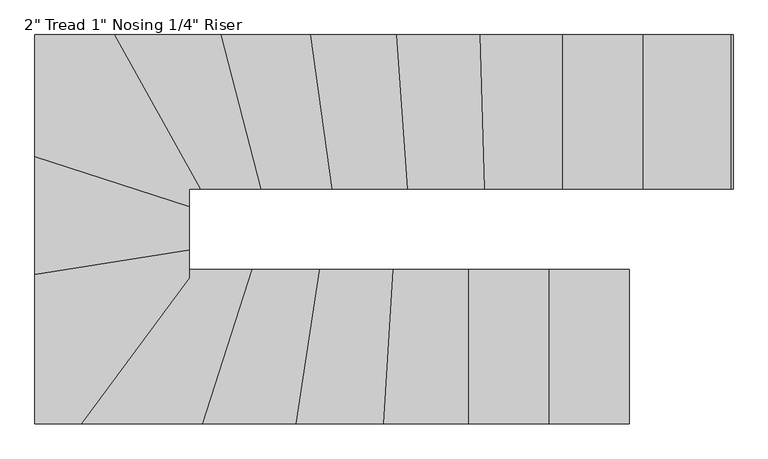
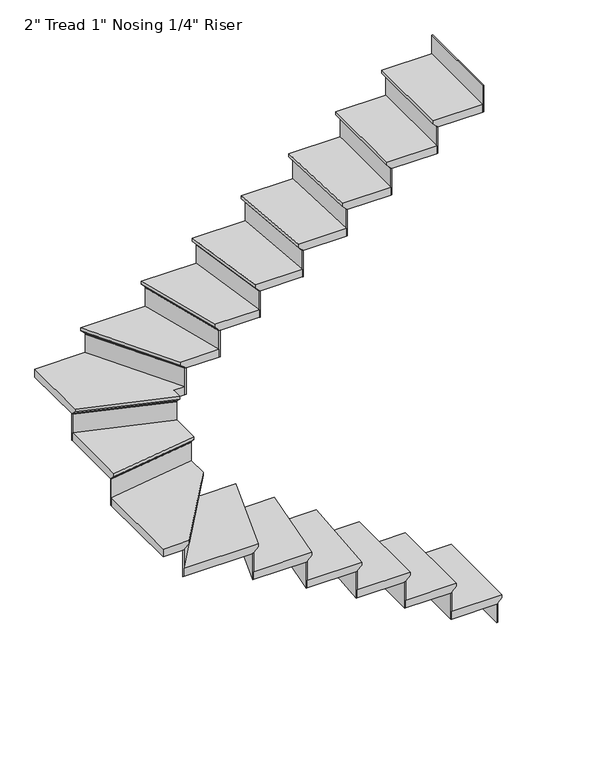
"""IFC4 building model written with IfcOpenShell, lengths in millimetres: stair flight geometry."""

from ifc_helpers import new_model, si_unit, origin, place, context, project, spatial, faceted_brep, source, transform, mapped, element, save


def stair_flight_0735e5f0(model_context):
    return source(origin(), model_context, "Body", "Brep", [
        faceted_brep([(-264.8831579, 264.4433073, 150.2833333), (-264.8831579, 264.4433073, 169.3333333), (-264.8831579, -271.8029286, 169.3333333), (-264.8831579, -271.8029286, 150.2833333), (-290.2831579, 264.4433073, 124.8833333), (-290.2831579, -271.8029286, 124.8833333), (-569.6831579, 264.4433073, 169.3333333), (-569.6831579, -271.8029286, 169.3333333), (-290.2831579, -271.8029286, 118.5333333), (-569.6831579, -271.8029286, 118.5333333), (-569.6831579, 264.4433073, 118.5333333), (-290.2831579, 264.4433073, 118.5333333)], [[[0, 1, 2, 3]], [[4, 0, 3, 5]], [[2, 1, 6, 7]], [[8, 9, 10, 11]], [[2, 7, 9, 8, 5, 3]], [[8, 11, 4, 5]], [[6, 1, 0, 4, 11, 10]], [[7, 6, 10, 9]]]),
        faceted_brep([(-290.2831579, 264.4433073, 118.5333333), (-290.2831579, 264.4433073, 0.0), (-296.6331579, 264.4433073, 0.0), (-296.6331579, 264.4433073, 118.5333333), (-290.2831579, -271.8029286, 118.5333333), (-296.6331579, -271.8029286, 118.5333333), (-296.6331579, -271.8029286, 0.0), (-290.2831579, -271.8029286, 0.0)], [[[0, 1, 2, 3]], [[4, 5, 6, 7]], [[1, 0, 4, 7]], [[2, 1, 7, 6]], [[3, 2, 6, 5]], [[0, 3, 5, 4]]]),
        faceted_brep([(-569.6831579, 264.4433073, 287.8666667), (-569.6831579, 264.4433073, 118.5333333), (-576.0331579, 264.4433073, 118.5333333), (-576.0331579, 264.4433073, 287.8666667), (-569.6831579, -271.8029286, 287.8666667), (-576.0331579, -271.8029286, 287.8666667), (-576.0331579, -271.8029286, 118.5333333), (-569.6831579, -271.8029286, 118.5333333)], [[[0, 1, 2, 3]], [[4, 5, 6, 7]], [[1, 0, 4, 7]], [[2, 1, 7, 6]], [[3, 2, 6, 5]], [[0, 3, 5, 4]]]),
        faceted_brep([(-544.2831579, -271.8029286, 338.6666667), (-544.2831579, 264.4433073, 338.6666667), (-849.0831579, 264.4433073, 338.6666667), (-849.0831579, -271.8029286, 338.6666667), (-569.6831579, -271.8029286, 287.8666667), (-849.0831579, -271.8029286, 287.8666667), (-849.0831579, 264.4433073, 287.8666667), (-569.6831579, 264.4433073, 287.8666667), (-569.6831579, -271.8029286, 294.2166667), (-544.2831579, -271.8029286, 319.6166667), (-569.6831579, 264.4433073, 294.2166667), (-544.2831579, 264.4433073, 319.6166667)], [[[0, 1, 2, 3]], [[4, 5, 6, 7]], [[0, 3, 5, 4, 8, 9]], [[4, 7, 10, 8]], [[2, 1, 11, 10, 7, 6]], [[3, 2, 6, 5]], [[11, 1, 0, 9]], [[10, 11, 9, 8]]]),
        faceted_brep([(-849.0831579, 264.4433073, 457.2), (-849.0831579, 264.4433073, 287.8666667), (-855.4331579, 264.4433073, 287.8666667), (-855.4331579, 264.4433073, 457.2), (-849.0831579, -271.8029286, 457.2), (-855.4331579, -271.8029286, 457.2), (-855.4331579, -271.8029286, 287.8666667), (-849.0831579, -271.8029286, 287.8666667)], [[[0, 1, 2, 3]], [[4, 5, 6, 7]], [[1, 0, 4, 7]], [[2, 1, 7, 6]], [[3, 2, 6, 5]], [[0, 3, 5, 4]]]),
        faceted_brep([(-823.6831579, -271.8029286, 508.0), (-823.6831579, 264.4433073, 508.0), (-1112.6009003, 264.4433073, 508.0), (-1144.4549627, -271.8029286, 508.0), (-849.0831579, -271.8029286, 457.2), (-1144.4549627, -271.8029286, 457.2), (-1112.6009003, 264.4433073, 457.2), (-849.0831579, 264.4433073, 457.2), (-849.0831579, -271.8029286, 463.55), (-823.6831579, -271.8029286, 488.95), (-849.0831579, 264.4433073, 463.55), (-823.6831579, 264.4433073, 488.95)], [[[0, 1, 2, 3]], [[4, 5, 6, 7]], [[0, 3, 5, 4, 8, 9]], [[4, 7, 10, 8]], [[2, 1, 11, 10, 7, 6]], [[3, 2, 6, 5]], [[11, 1, 0, 9]], [[10, 11, 9, 8]]]),
        faceted_brep([(-1112.6009003, 264.4433073, 626.5333333), (-1112.6009003, 264.4433073, 457.2), (-1118.9620938, 264.4433073, 457.2), (-1118.9620938, 264.4433073, 626.5333333), (-1144.4549627, -271.8029286, 626.5333333), (-1150.8161561, -271.8029286, 626.5333333), (-1150.8161561, -271.8029286, 457.2), (-1144.4549627, -271.8029286, 457.2)], [[[0, 1, 2, 3]], [[4, 5, 6, 7]], [[1, 0, 4, 7]], [[2, 1, 7, 6]], [[3, 2, 6, 5]], [[0, 3, 5, 4]]]),
        faceted_brep([(-1119.0101891, -271.8029286, 677.3333333), (-1087.1561267, 264.4433073, 677.3333333), (-1367.1376579, 264.4433073, 677.3333333), (-1449.2203373, -271.8029286, 677.3333333), (-1144.4549627, -271.8029286, 626.5333333), (-1449.2203373, -271.8029286, 626.5333333), (-1367.1376579, 264.4433073, 626.5333333), (-1112.6009003, 264.4433073, 626.5333333), (-1144.4549627, -271.8029286, 632.8833333), (-1119.0101891, -271.8029286, 658.2833333), (-1112.6009003, 264.4433073, 632.8833333), (-1087.1561267, 264.4433073, 658.2833333)], [[[0, 1, 2, 3]], [[4, 5, 6, 7]], [[0, 3, 5, 4, 8, 9]], [[4, 7, 10, 8]], [[2, 1, 11, 10, 7, 6]], [[3, 2, 6, 5]], [[11, 1, 0, 9]], [[10, 11, 9, 8]]]),
        faceted_brep([(-1367.1376579, 264.4433073, 795.8666667), (-1367.1376579, 264.4433073, 626.5333333), (-1373.5616178, 264.4433073, 626.5333333), (-1373.5616178, 264.4433073, 795.8666667), (-1449.2203373, -271.8029286, 795.8666667), (-1455.6442972, -271.8029286, 795.8666667), (-1455.6442972, -271.8029286, 626.5333333), (-1449.2203373, -271.8029286, 626.5333333)], [[[0, 1, 2, 3]], [[4, 5, 6, 7]], [[1, 0, 4, 7]], [[2, 1, 7, 6]], [[3, 2, 6, 5]], [[0, 3, 5, 4]]]),
        faceted_brep([(-1423.5244976, -271.8029286, 846.6666667), (-1341.4418182, 264.4433073, 846.6666667), (-1602.0584075, 264.4433073, 846.6666667), (-1775.0869242, -271.8029286, 846.6666667), (-1449.2203373, -271.8029286, 795.8666667), (-1775.0869242, -271.8029286, 795.8666667), (-1602.0584075, 264.4433073, 795.8666667), (-1367.1376579, 264.4433073, 795.8666667), (-1449.2203373, -271.8029286, 802.2166667), (-1423.5244976, -271.8029286, 827.6166667), (-1367.1376579, 264.4433073, 802.2166667), (-1341.4418182, 264.4433073, 827.6166667)], [[[0, 1, 2, 3]], [[4, 5, 6, 7]], [[0, 3, 5, 4, 8, 9]], [[4, 7, 10, 8]], [[2, 1, 11, 10, 7, 6]], [[3, 2, 6, 5]], [[11, 1, 0, 9]], [[10, 11, 9, 8]]]),
        faceted_brep([(-1602.0584075, 264.4433073, 965.2), (-1602.0584075, 264.4433073, 795.8666667), (-1608.7307845, 264.4433073, 795.8666667), (-1608.7307845, 264.4433073, 965.2), (-1775.0869242, -271.8029286, 965.2), (-1781.7593012, -271.8029286, 965.2), (-1781.7593012, -271.8029286, 795.8666667), (-1775.0869242, -271.8029286, 795.8666667)], [[[0, 1, 2, 3]], [[4, 5, 6, 7]], [[1, 0, 4, 7]], [[2, 1, 7, 6]], [[3, 2, 6, 5]], [[0, 3, 5, 4]]]),
        faceted_brep([(-1748.3974163, -271.8029286, 1016.0), (-1575.3688995, 264.4433073, 1016.0), (-1792.6148498, 264.4433073, 1016.0), (-1792.6148498, 277.721026, 1016.0), (-2200.2950016, -271.8029286, 1016.0), (-1775.0869242, -271.8029286, 965.2), (-2200.2950016, -271.8029286, 965.2), (-1792.6148498, 277.721026, 965.2), (-1792.6148498, 264.4433073, 965.2), (-1602.0584075, 264.4433073, 965.2), (-1775.0869242, -271.8029286, 971.55), (-1748.3974163, -271.8029286, 996.95), (-1602.0584075, 264.4433073, 971.55), (-1575.3688995, 264.4433073, 996.95)], [[[0, 1, 2, 3, 4]], [[5, 6, 7, 8, 9]], [[0, 4, 6, 5, 10, 11]], [[5, 9, 12, 10]], [[2, 1, 13, 12, 9, 8]], [[4, 3, 7, 6]], [[13, 1, 0, 11]], [[12, 13, 11, 10]], [[3, 2, 8, 7]]]),
        faceted_brep([(-1792.6148498, 277.721026, 1134.5333333), (-1792.6148498, 277.721026, 965.2), (-1792.6148498, 288.3786511, 965.2), (-1792.6148498, 288.3786511, 1134.5333333), (-2200.2950016, -271.8029286, 1134.5333333), (-2208.2016673, -271.8029286, 1134.5333333), (-2208.2016673, -271.8029286, 965.2), (-2200.2950016, -271.8029286, 965.2)], [[[0, 1, 2, 3]], [[4, 5, 6, 7]], [[1, 0, 4, 7]], [[2, 1, 7, 6]], [[3, 2, 6, 5]], [[0, 3, 5, 4]]]),
        faceted_brep([(-2328.8610857, 272.9225747, 1185.3333333), (-2328.8610857, -271.8029286, 1185.3333333), (-2168.6683387, -271.8029286, 1185.3333333), (-1792.6148498, 235.0905257, 1185.3333333), (-1792.6148498, 358.7948785, 1185.3333333), (-2328.8610857, -271.8029286, 1134.5333333), (-2328.8610857, 272.9225747, 1134.5333333), (-1792.6148498, 358.7948785, 1134.5333333), (-1792.6148498, 277.721026, 1134.5333333), (-2200.2950016, -271.8029286, 1134.5333333), (-2200.2950016, -271.8029286, 1140.8833333), (-2168.6683387, -271.8029286, 1166.2833333), (-1792.6148498, 277.721026, 1140.8833333), (-1792.6148498, 235.0905257, 1166.2833333)], [[[0, 1, 2, 3, 4]], [[5, 6, 7, 8, 9]], [[1, 0, 6, 5]], [[2, 1, 5, 9, 10, 11]], [[9, 8, 12, 10]], [[4, 3, 13, 12, 8, 7]], [[0, 4, 7, 6]], [[13, 3, 2, 11]], [[12, 13, 11, 10]]]),
        faceted_brep([(-1792.6148498, 358.7948785, 1303.8666667), (-1792.6148498, 358.7948785, 1134.5333333), (-1792.6148498, 365.2257813, 1134.5333333), (-1792.6148498, 365.2257813, 1303.8666667), (-2328.8610857, 272.9225747, 1303.8666667), (-2328.8610857, 279.3534775, 1303.8666667), (-2328.8610857, 279.3534775, 1134.5333333), (-2328.8610857, 272.9225747, 1134.5333333)], [[[0, 1, 2, 3]], [[4, 5, 6, 7]], [[1, 0, 4, 7]], [[2, 1, 7, 6]], [[3, 2, 6, 5]], [[0, 3, 5, 4]]]),
        faceted_brep([(-2328.8610857, 247.1989634, 1354.6666667), (-1792.6148498, 333.0712672, 1354.6666667), (-1792.6148498, 510.0383883, 1354.6666667), (-2328.8610857, 683.2061106, 1354.6666667), (-2328.8610857, 272.9225747, 1303.8666667), (-2328.8610857, 683.2061106, 1303.8666667), (-1792.6148498, 510.0383883, 1303.8666667), (-1792.6148498, 358.7948785, 1303.8666667), (-2328.8610857, 272.9225747, 1310.2166667), (-2328.8610857, 247.1989634, 1335.6166667), (-1792.6148498, 358.7948785, 1310.2166667), (-1792.6148498, 333.0712672, 1335.6166667)], [[[0, 1, 2, 3]], [[4, 5, 6, 7]], [[0, 3, 5, 4, 8, 9]], [[4, 7, 10, 8]], [[3, 2, 6, 5]], [[11, 1, 0, 9]], [[10, 11, 9, 8]], [[2, 1, 11, 10, 7, 6]]]),
        faceted_brep([(-1792.6148498, 510.0383883, 1473.2), (-1792.6148498, 510.0383883, 1303.8666667), (-1792.6148498, 516.7112716, 1303.8666667), (-1792.6148498, 516.7112716, 1473.2), (-2328.8610857, 683.2061106, 1473.2), (-2328.8610857, 689.878994, 1473.2), (-2328.8610857, 689.878994, 1303.8666667), (-2328.8610857, 683.2061106, 1303.8666667)], [[[0, 1, 2, 3]], [[4, 5, 6, 7]], [[1, 0, 4, 7]], [[2, 1, 7, 6]], [[3, 2, 6, 5]], [[0, 3, 5, 4]]]),
        faceted_brep([(-2021.9568272, 1080.0895433, 1524.0), (-2328.8610857, 1080.0895433, 1524.0), (-2328.8610857, 656.5145772, 1524.0), (-1792.6148498, 483.3468548, 1524.0), (-1792.6148498, 543.8433073, 1524.0), (-1724.5287393, 543.8433073, 1524.0), (-2328.8610857, 1080.0895433, 1473.2), (-2021.9568272, 1080.0895433, 1473.2), (-1724.5287393, 543.8433073, 1473.2), (-1792.6148498, 543.8433073, 1473.2), (-1792.6148498, 510.0383883, 1473.2), (-2328.8610857, 683.2061106, 1473.2), (-1792.6148498, 510.0383883, 1479.55), (-2328.8610857, 683.2061106, 1479.55), (-1792.6148498, 483.3468548, 1504.95), (-2328.8610857, 656.5145772, 1504.95)], [[[0, 1, 2, 3, 4, 5]], [[6, 7, 8, 9, 10, 11]], [[1, 0, 7, 6]], [[11, 10, 12, 13]], [[4, 3, 14, 12, 10, 9]], [[0, 5, 8, 7]], [[14, 3, 2, 15]], [[12, 14, 15, 13]], [[2, 1, 6, 11, 13, 15]], [[5, 4, 9, 8]]]),
        faceted_brep([(-1724.5287393, 543.8433073, 1642.5333333), (-1724.5287393, 543.8433073, 1473.2), (-1717.2673962, 543.8433073, 1473.2), (-1717.2673962, 543.8433073, 1642.5333333), (-2021.9568272, 1080.0895433, 1642.5333333), (-2014.6954841, 1080.0895433, 1642.5333333), (-2014.6954841, 1080.0895433, 1473.2), (-2021.9568272, 1080.0895433, 1473.2)], [[[0, 1, 2, 3]], [[4, 5, 6, 7]], [[1, 0, 4, 7]], [[2, 1, 7, 6]], [[3, 2, 6, 5]], [[0, 3, 5, 4]]]),
        faceted_brep([(-2051.0021996, 1080.0895433, 1693.3333333), (-1753.5741117, 543.8433073, 1693.3333333), (-1517.487325, 543.8433073, 1693.3333333), (-1656.0375972, 1080.0895433, 1693.3333333), (-2021.9568272, 1080.0895433, 1642.5333333), (-1656.0375972, 1080.0895433, 1642.5333333), (-1517.487325, 543.8433073, 1642.5333333), (-1724.5287393, 543.8433073, 1642.5333333), (-2021.9568272, 1080.0895433, 1648.8833333), (-2051.0021996, 1080.0895433, 1674.2833333), (-1724.5287393, 543.8433073, 1648.8833333), (-1753.5741117, 543.8433073, 1674.2833333)], [[[0, 1, 2, 3]], [[4, 5, 6, 7]], [[0, 3, 5, 4, 8, 9]], [[4, 7, 10, 8]], [[2, 1, 11, 10, 7, 6]], [[3, 2, 6, 5]], [[11, 1, 0, 9]], [[10, 11, 9, 8]]]),
        faceted_brep([(-1517.487325, 543.8433073, 1811.8666667), (-1517.487325, 543.8433073, 1642.5333333), (-1510.9288005, 543.8433073, 1642.5333333), (-1510.9288005, 543.8433073, 1811.8666667), (-1656.0375972, 1080.0895433, 1811.8666667), (-1649.4790727, 1080.0895433, 1811.8666667), (-1649.4790727, 1080.0895433, 1642.5333333), (-1656.0375972, 1080.0895433, 1642.5333333)], [[[0, 1, 2, 3]], [[4, 5, 6, 7]], [[1, 0, 4, 7]], [[2, 1, 7, 6]], [[3, 2, 6, 5]], [[0, 3, 5, 4]]]),
        faceted_brep([(-1682.2716952, 1080.0895433, 1862.6666667), (-1543.721423, 543.8433073, 1862.6666667), (-1271.2041837, 543.8433073, 1862.6666667), (-1344.713853, 1080.0895433, 1862.6666667), (-1656.0375972, 1080.0895433, 1811.8666667), (-1344.713853, 1080.0895433, 1811.8666667), (-1271.2041837, 543.8433073, 1811.8666667), (-1517.487325, 543.8433073, 1811.8666667), (-1656.0375972, 1080.0895433, 1818.2166667), (-1682.2716952, 1080.0895433, 1843.6166667), (-1517.487325, 543.8433073, 1818.2166667), (-1543.721423, 543.8433073, 1843.6166667)], [[[0, 1, 2, 3]], [[4, 5, 6, 7]], [[0, 3, 5, 4, 8, 9]], [[4, 7, 10, 8]], [[2, 1, 11, 10, 7, 6]], [[3, 2, 6, 5]], [[11, 1, 0, 9]], [[10, 11, 9, 8]]]),
        faceted_brep([(-1271.2041837, 543.8433073, 1981.2), (-1271.2041837, 543.8433073, 1811.8666667), (-1264.7947985, 543.8433073, 1811.8666667), (-1264.7947985, 543.8433073, 1981.2), (-1344.713853, 1080.0895433, 1981.2), (-1338.3044678, 1080.0895433, 1981.2), (-1338.3044678, 1080.0895433, 1811.8666667), (-1344.713853, 1080.0895433, 1811.8666667)], [[[0, 1, 2, 3]], [[4, 5, 6, 7]], [[1, 0, 4, 7]], [[2, 1, 7, 6]], [[3, 2, 6, 5]], [[0, 3, 5, 4]]]),
        faceted_brep([(-1370.3513937, 1080.0895433, 2032.0), (-1296.8417245, 543.8433073, 2032.0), (-1009.7763573, 543.8433073, 2032.0), (-1047.6899509, 1080.0895433, 2032.0), (-1344.713853, 1080.0895433, 1981.2), (-1047.6899509, 1080.0895433, 1981.2), (-1009.7763573, 543.8433073, 1981.2), (-1271.2041837, 543.8433073, 1981.2), (-1344.713853, 1080.0895433, 1987.55), (-1370.3513937, 1080.0895433, 2012.95), (-1271.2041837, 543.8433073, 1987.55), (-1296.8417245, 543.8433073, 2012.95)], [[[0, 1, 2, 3]], [[4, 5, 6, 7]], [[0, 3, 5, 4, 8, 9]], [[4, 7, 10, 8]], [[2, 1, 11, 10, 7, 6]], [[3, 2, 6, 5]], [[11, 1, 0, 9]], [[10, 11, 9, 8]]]),
        faceted_brep([(-1009.7763573, 543.8433073, 2150.5333333), (-1009.7763573, 543.8433073, 1981.2), (-1003.4105061, 543.8433073, 1981.2), (-1003.4105061, 543.8433073, 2150.5333333), (-1047.6899509, 1080.0895433, 2150.5333333), (-1041.3240997, 1080.0895433, 2150.5333333), (-1041.3240997, 1080.0895433, 1981.2), (-1047.6899509, 1080.0895433, 1981.2)], [[[0, 1, 2, 3]], [[4, 5, 6, 7]], [[1, 0, 4, 7]], [[2, 1, 7, 6]], [[3, 2, 6, 5]], [[0, 3, 5, 4]]]),
        faceted_brep([(-1073.1533559, 1080.0895433, 2201.3333333), (-1035.2397623, 543.8433073, 2201.3333333), (-741.6570892, 543.8433073, 2201.3333333), (-757.1149275, 1080.0895433, 2201.3333333), (-1047.6899509, 1080.0895433, 2150.5333333), (-757.1149275, 1080.0895433, 2150.5333333), (-741.6570892, 543.8433073, 2150.5333333), (-1009.7763573, 543.8433073, 2150.5333333), (-1047.6899509, 1080.0895433, 2156.8833333), (-1073.1533559, 1080.0895433, 2182.2833333), (-1009.7763573, 543.8433073, 2156.8833333), (-1035.2397623, 543.8433073, 2182.2833333)], [[[0, 1, 2, 3]], [[4, 5, 6, 7]], [[0, 3, 5, 4, 8, 9]], [[4, 7, 10, 8]], [[2, 1, 11, 10, 7, 6]], [[3, 2, 6, 5]], [[11, 1, 0, 9]], [[10, 11, 9, 8]]]),
        faceted_brep([(-741.6570892, 543.8433073, 2319.8666667), (-741.6570892, 543.8433073, 2150.5333333), (-735.3044516, 543.8433073, 2150.5333333), (-735.3044516, 543.8433073, 2319.8666667), (-757.1149275, 1080.0895433, 2319.8666667), (-750.7622898, 1080.0895433, 2319.8666667), (-750.7622898, 1080.0895433, 2150.5333333), (-757.1149275, 1080.0895433, 2150.5333333)], [[[0, 1, 2, 3]], [[4, 5, 6, 7]], [[1, 0, 4, 7]], [[2, 1, 7, 6]], [[3, 2, 6, 5]], [[0, 3, 5, 4]]]),
        faceted_brep([(-782.5254783, 1080.0895433, 2370.6666667), (-767.06764, 543.8433073, 2370.6666667), (-469.9965591, 543.8433073, 2370.6666667), (-469.9965591, 1080.0895433, 2370.6666667), (-757.1149275, 1080.0895433, 2319.8666667), (-469.9965591, 1080.0895433, 2319.8666667), (-469.9965591, 543.8433073, 2319.8666667), (-741.6570892, 543.8433073, 2319.8666667), (-757.1149275, 1080.0895433, 2326.2166667), (-782.5254783, 1080.0895433, 2351.6166667), (-741.6570892, 543.8433073, 2326.2166667), (-767.06764, 543.8433073, 2351.6166667)], [[[0, 1, 2, 3]], [[4, 5, 6, 7]], [[0, 3, 5, 4, 8, 9]], [[4, 7, 10, 8]], [[2, 1, 11, 10, 7, 6]], [[3, 2, 6, 5]], [[11, 1, 0, 9]], [[10, 11, 9, 8]]]),
        faceted_brep([(-469.9965591, 543.8433073, 2489.2), (-469.9965591, 543.8433073, 2319.8666667), (-463.6465591, 543.8433073, 2319.8666667), (-463.6465591, 543.8433073, 2489.2), (-469.9965591, 1080.0895433, 2489.2), (-463.6465591, 1080.0895433, 2489.2), (-463.6465591, 1080.0895433, 2319.8666667), (-469.9965591, 1080.0895433, 2319.8666667)], [[[0, 1, 2, 3]], [[4, 5, 6, 7]], [[1, 0, 4, 7]], [[2, 1, 7, 6]], [[3, 2, 6, 5]], [[0, 3, 5, 4]]]),
        faceted_brep([(-495.3965591, 1080.0895433, 2540.0), (-495.3965591, 543.8433073, 2540.0), (-190.5965591, 543.8433073, 2540.0), (-190.5965591, 1080.0895433, 2540.0), (-469.9965591, 1080.0895433, 2489.2), (-190.5965591, 1080.0895433, 2489.2), (-190.5965591, 543.8433073, 2489.2), (-469.9965591, 543.8433073, 2489.2), (-469.9965591, 1080.0895433, 2495.55), (-495.3965591, 1080.0895433, 2520.95), (-469.9965591, 543.8433073, 2495.55), (-495.3965591, 543.8433073, 2520.95)], [[[0, 1, 2, 3]], [[4, 5, 6, 7]], [[0, 3, 5, 4, 8, 9]], [[4, 7, 10, 8]], [[2, 1, 11, 10, 7, 6]], [[3, 2, 6, 5]], [[11, 1, 0, 9]], [[10, 11, 9, 8]]]),
        faceted_brep([(-190.5965591, 543.8433073, 2658.5333333), (-190.5965591, 543.8433073, 2489.2), (-184.2465591, 543.8433073, 2489.2), (-184.2465591, 543.8433073, 2658.5333333), (-190.5965591, 1080.0895433, 2658.5333333), (-184.2465591, 1080.0895433, 2658.5333333), (-184.2465591, 1080.0895433, 2489.2), (-190.5965591, 1080.0895433, 2489.2)], [[[0, 1, 2, 3]], [[4, 5, 6, 7]], [[1, 0, 4, 7]], [[2, 1, 7, 6]], [[3, 2, 6, 5]], [[0, 3, 5, 4]]]),
        faceted_brep([(88.8034409, 543.8433073, 2827.8666667), (88.8034409, 543.8433073, 2658.5333333), (95.1534409, 543.8433073, 2658.5333333), (95.1534409, 543.8433073, 2827.8666667), (88.8034409, 1080.0895433, 2827.8666667), (95.1534409, 1080.0895433, 2827.8666667), (95.1534409, 1080.0895433, 2658.5333333), (88.8034409, 1080.0895433, 2658.5333333)], [[[0, 1, 2, 3]], [[4, 5, 6, 7]], [[1, 0, 4, 7]], [[2, 1, 7, 6]], [[3, 2, 6, 5]], [[0, 3, 5, 4]]]),
        faceted_brep([(-215.9965591, 1080.0895433, 2709.3333333), (-215.9965591, 543.8433073, 2709.3333333), (88.8034409, 543.8433073, 2709.3333333), (88.8034409, 1080.0895433, 2709.3333333), (-190.5965591, 1080.0895433, 2658.5333333), (88.8034409, 1080.0895433, 2658.5333333), (88.8034409, 543.8433073, 2658.5333333), (-190.5965591, 543.8433073, 2658.5333333), (-190.5965591, 1080.0895433, 2664.8833333), (-215.9965591, 1080.0895433, 2690.2833333), (-190.5965591, 543.8433073, 2664.8833333), (-215.9965591, 543.8433073, 2690.2833333)], [[[0, 1, 2, 3]], [[4, 5, 6, 7]], [[0, 3, 5, 4, 8, 9]], [[4, 7, 10, 8]], [[2, 1, 11, 10, 7, 6]], [[3, 2, 6, 5]], [[11, 1, 0, 9]], [[10, 11, 9, 8]]]),
    ])


if __name__ == "__main__":
    model = new_model("IFC4")
    model_context = context("Model", 3, world=origin())
    ifc_project = project(units=[si_unit("LENGTHUNIT", "METRE", prefix="MILLI")], contexts=[model_context])
    site = spatial("IfcSite", under=ifc_project)
    building = spatial("IfcBuilding", under=site)
    placement = place(None, origin())
    stair_flight_shape = stair_flight_0735e5f0(model_context)
    element("IfcStairFlight", 1, ObjectType="2\" Tread 1\" Nosing 1/4\" Riser", at=placement, inside=building, context=model_context, shape_type="MappedRepresentation", body=[
        mapped(stair_flight_shape, transform((0.0, 0.0, 0.0), x_axis=(1.0, 0.0, 0.0), y_axis=(0.0, 1.0, 0.0), z_axis=(0.0, 0.0, 1.0))),
    ])
    save(model, "model.ifc")
